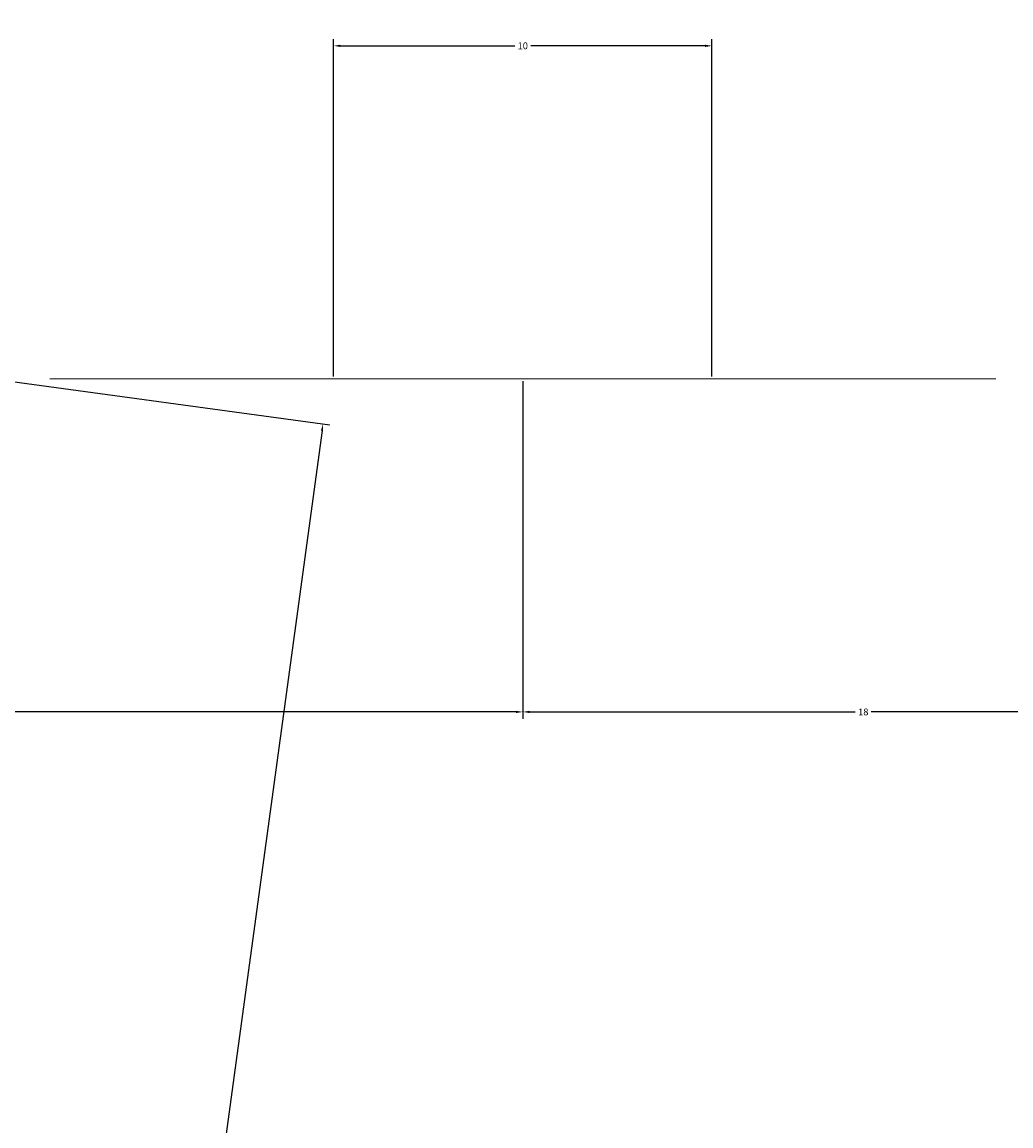
# Model space of a CAD drawing. Units: millimetres. Extents: x -9 to 135, y -119 to 27.
# Tile 10 of 12: x 95 to 121, y -18 to 11. Entities that reach past the tile are written whole.
import ezdxf

# ---------------------------------------------------------------- set-up
doc = ezdxf.new("R2010")
doc.units = ezdxf.units.MM
doc.layers.add('M-CONS', color=8, linetype='Continuous', lineweight=18)
doc.layers.add('M-DIMS', color=2, linetype='Continuous', lineweight=18)
doc.styles.get("Standard").update_dxf_attribs({"font": 'arial.ttf'})
doc.dimstyles.get("Standard").update_dxf_attribs({"dimtxt": 0.18, "dimasz": 0.18, "dimexe": 0.18, "dimexo": 0.0625, "dimgap": 0.09, "dimtad": 0, "dimtih": 1, "dimtoh": 1, "dimdec": 4, "dimzin": 0, "dimdsep": 46, "dimtxsty": 'Standard', "dimcen": 0.09, "dimadec": 0, "dimazin": 0, "dimtfac": 1, "dimtdec": 4, "dimtofl": 0, "dimtmove": 0, "dimatfit": 3, "dimfxl": 1, "dimtolj": 1, "dimtzin": 0, "dimarcsym": 0})

# ---------------------------------------------------------------- blocks, each defined once
blk = doc.blocks.new('BOSS-PROFILE-D25-BORE10')
at = {"extrusion": (0, -1, 0)}
for radius in [12.5, 5]:
    blk.add_circle((12.5, 101.129, 0), radius, dxfattribs=at)
blk = doc.blocks.new('*D2')
at = {"layer": 'Defpoints', "color": 0, "transparency": 16777216}
for p in [(126, 26.533), (0, 17.733), (126, 1.733)]:
    blk.add_point(p, dxfattribs=at)
at = {"layer": 'M-DIMS', "color": 0, "lineweight": -2, "transparency": 16777216}
for p, q in [((0, 17.796), (0, 26.713)), ((126, 1.796), (126, 26.713)), ((0.18, 26.533), (62.72, 26.533)), ((125.82, 26.533), (63.28, 26.533))]:
    blk.add_line(p, q, dxfattribs=at)
at = {"layer": 'M-DIMS', "color": 0, "transparency": 16777216}
for points in [[(0.18, 26.563), (0.18, 26.503), (0, 26.533)], [(125.82, 26.563), (125.82, 26.503), (126, 26.533)]]:
    blk.add_solid(points, dxfattribs=at)
at = {"layer": 'M-DIMS', "color": 0, "transparency": 16777216, "insert": (63, 26.533), "char_height": 0.18, "attachment_point": 5}
blk.add_mtext('\\A1;126', dxfattribs=at)
blk = doc.blocks.new('*D7')
at = {"layer": 'Defpoints', "color": 0, "transparency": 16777216}
for p in [(113, 10.533), (103, 1.733), (113, 1.733)]:
    blk.add_point(p, dxfattribs=at)
at = {"layer": 'M-DIMS', "color": 0, "lineweight": -2, "transparency": 16777216}
for p, q in [((103, 1.796), (103, 10.713)), ((103.18, 10.533), (107.79, 10.533)), ((112.82, 10.533), (108.21, 10.533)), ((113, 1.796), (113, 10.713))]:
    blk.add_line(p, q, dxfattribs=at)
at = {"layer": 'M-DIMS', "color": 0, "transparency": 16777216}
for points in [[(103.18, 10.563), (103.18, 10.503), (103, 10.533)], [(112.82, 10.563), (112.82, 10.503), (113, 10.533)]]:
    blk.add_solid(points, dxfattribs=at)
at = {"layer": 'M-DIMS', "color": 0, "transparency": 16777216, "insert": (108, 10.533), "char_height": 0.18, "attachment_point": 5}
blk.add_mtext('\\A1;10', dxfattribs=at)
blk = doc.blocks.new('*D10')
at = {"layer": 'Defpoints', "color": 0, "transparency": 16777216}
for p in [(63, 1.733), (108, 1.733), (63, -7.067)]:
    blk.add_point(p, dxfattribs=at)
at = {"layer": 'M-DIMS', "color": 0, "lineweight": -2, "transparency": 16777216}
for p, q in [((63, 1.671), (63, -7.247)), ((108, 1.671), (108, -7.247)), ((63.18, -7.067), (85.277, -7.067)), ((107.82, -7.067), (85.723, -7.067))]:
    blk.add_line(p, q, dxfattribs=at)
at = {"layer": 'M-DIMS', "color": 0, "transparency": 16777216}
for points in [[(63.18, -7.037), (63.18, -7.097), (63, -7.067)], [(107.82, -7.037), (107.82, -7.097), (108, -7.067)]]:
    blk.add_solid(points, dxfattribs=at)
at = {"layer": 'M-DIMS', "color": 0, "transparency": 16777216, "insert": (85.5, -7.067), "char_height": 0.18, "attachment_point": 5}
blk.add_mtext('\\A1;45', dxfattribs=at)
blk = doc.blocks.new('*D11')
at = {"layer": 'Defpoints', "color": 0, "transparency": 16777216}
for p in [(108, 1.733), (126, 1.733), (108, -7.067)]:
    blk.add_point(p, dxfattribs=at)
at = {"layer": 'M-DIMS', "color": 0, "lineweight": -2, "transparency": 16777216}
for p, q in [((108, 1.671), (108, -7.247)), ((126, 1.671), (126, -7.247)), ((108.18, -7.067), (116.789, -7.067)), ((125.82, -7.067), (117.211, -7.067))]:
    blk.add_line(p, q, dxfattribs=at)
at = {"layer": 'M-DIMS', "color": 0, "transparency": 16777216}
for points in [[(108.18, -7.037), (108.18, -7.097), (108, -7.067)], [(125.82, -7.037), (125.82, -7.097), (126, -7.067)]]:
    blk.add_solid(points, dxfattribs=at)
at = {"layer": 'M-DIMS', "color": 0, "transparency": 16777216, "insert": (117, -7.067), "char_height": 0.18, "attachment_point": 5}
blk.add_mtext('\\A1;18', dxfattribs=at)
blk = doc.blocks.new('*D13')
at = {"layer": 'Defpoints', "color": 0, "transparency": 16777216}
for p in [(126, 1.733), (63, -92.267), (134.8, -92.267)]:
    blk.add_point(p, dxfattribs=at)
at = {"layer": 'M-DIMS', "color": 0, "lineweight": -2, "transparency": 16777216}
for p, q in [((126.062, 1.733), (134.98, 1.733)), ((134.8, 1.553), (134.8, -45.085)), ((134.8, -92.087), (134.8, -45.449)), ((63.063, -92.267), (134.98, -92.267))]:
    blk.add_line(p, q, dxfattribs=at)
at = {"layer": 'M-DIMS', "color": 0, "transparency": 16777216}
for points in [[(134.77, 1.553), (134.83, 1.553), (134.8, 1.733)], [(134.77, -92.087), (134.83, -92.087), (134.8, -92.267)]]:
    blk.add_solid(points, dxfattribs=at)
at = {"layer": 'M-DIMS', "color": 0, "transparency": 16777216, "insert": (134.8, -45.267), "char_height": 0.18, "attachment_point": 5}
blk.add_mtext('\\A1;94', dxfattribs=at)
blk = doc.blocks.new('*D15')
at = {"layer": 'Defpoints', "color": 0, "transparency": 16777216}
for p in [(94, 1.733), (80.835, -94.702), (89.554, -95.892)]:
    blk.add_point(p, dxfattribs=at)
at = {"layer": 'M-DIMS', "color": 0, "lineweight": -2, "transparency": 16777216}
for p, q in [((94.062, 1.725), (102.897, 0.519)), ((102.695, 0.365), (96.161, -47.493)), ((89.578, -95.714), (96.112, -47.856)), ((80.896, -94.71), (89.732, -95.916))]:
    blk.add_line(p, q, dxfattribs=at)
at = {"layer": 'M-DIMS', "color": 0, "transparency": 16777216}
for points in [[(102.665, 0.369), (102.724, 0.36), (102.719, 0.543)], [(89.548, -95.71), (89.608, -95.718), (89.554, -95.892)]]:
    blk.add_solid(points, dxfattribs=at)
at = {"layer": 'M-DIMS', "color": 0, "transparency": 16777216, "insert": (96.136, -47.675), "char_height": 0.18, "attachment_point": 5}
blk.add_mtext('\\A1;97.33', dxfattribs=at)
blk = doc.blocks.new('*D16')
at = {"layer": 'Defpoints', "color": 0, "transparency": 16777216}
for p in [(126, 1.733), (63, -92.267), (126, -119.067)]:
    blk.add_point(p, dxfattribs=at)
at = {"layer": 'M-DIMS', "color": 0, "lineweight": -2, "transparency": 16777216}
for p, q in [((126, 1.671), (126, -119.247)), ((63, -92.329), (63, -119.247)), ((63.18, -119.067), (94.281, -119.067)), ((125.82, -119.067), (94.719, -119.067))]:
    blk.add_line(p, q, dxfattribs=at)
at = {"layer": 'M-DIMS', "color": 0, "transparency": 16777216}
for points in [[(63.18, -119.037), (63.18, -119.097), (63, -119.067)], [(125.82, -119.037), (125.82, -119.097), (126, -119.067)]]:
    blk.add_solid(points, dxfattribs=at)
at = {"layer": 'M-DIMS', "color": 0, "transparency": 16777216, "insert": (94.5, -119.067), "char_height": 0.18, "attachment_point": 5}
blk.add_mtext('\\A1;63', dxfattribs=at)

msp = doc.modelspace()

# ---------------------------------------------------------------- block references
at = {"layer": 'M-CONS'}
msp.add_blockref('BOSS-PROFILE-D25-BORE10', (95.5, 1.733), dxfattribs=at)

# ---------------------------------------------------------------- dimensions: what is measured, and where the dimension line sits
at = {"layer": 'M-DIMS'}
for base, p1, p2, picture, middle in [((126, 26.533), (0, 17.733), (126, 1.733), '*D2', (63, 26.533)), ((113, 10.533), (103, 1.733), (113, 1.733), '*D7', (108, 10.533)), ((126, -119.067), (63, -92.267), (126, 1.733), '*D16', (94.5, -119.067))]:
    dim = msp.add_linear_dim(base=base, p1=p1, p2=p2, dimstyle='Standard', override={"dimdec": 0, "dimlfac": 1, "dimrnd": 0, "dimzin": 0, "dimdsep": 46, "dimlunit": 2}, dxfattribs=at)
    dim.commit()
    dim.dimension.update_dxf_attribs({"geometry": picture, "text_midpoint": middle})
for base, p1, p2, angle, override, picture, middle in [((63, -7.067), (108, 1.733), (63, 1.733), 180, {"dimdec": 0, "dimlfac": 1, "dimrnd": 0, "dimzin": 0, "dimdsep": 46, "dimlunit": 2}, '*D10', (85.5, -7.067)), ((134.8, -92.267), (126, 1.733), (63, -92.267), 90, {"dimdec": 0, "dimlfac": 1, "dimrnd": 0, "dimzin": 0, "dimdsep": 46, "dimlunit": 2}, '*D13', (134.8, -45.267)), ((89.554, -95.892), (94, 1.733), (80.835, -94.702), 262.2259, {"dimdec": 2, "dimlfac": 1, "dimrnd": 0, "dimzin": 0, "dimdsep": 46, "dimlunit": 2}, '*D15', (96.136, -47.675)), ((108, -7.067), (126, 1.733), (108, 1.733), 180, {"dimdec": 0, "dimlfac": 1, "dimrnd": 0, "dimzin": 0, "dimdsep": 46, "dimlunit": 2}, '*D11', (117, -7.067))]:
    dim = msp.add_linear_dim(base=base, p1=p1, p2=p2, angle=angle, dimstyle='Standard', override=override, dxfattribs=at)
    dim.commit()
    dim.dimension.update_dxf_attribs({"geometry": picture, "text_midpoint": middle})

doc.saveas('drawing.dxf')
